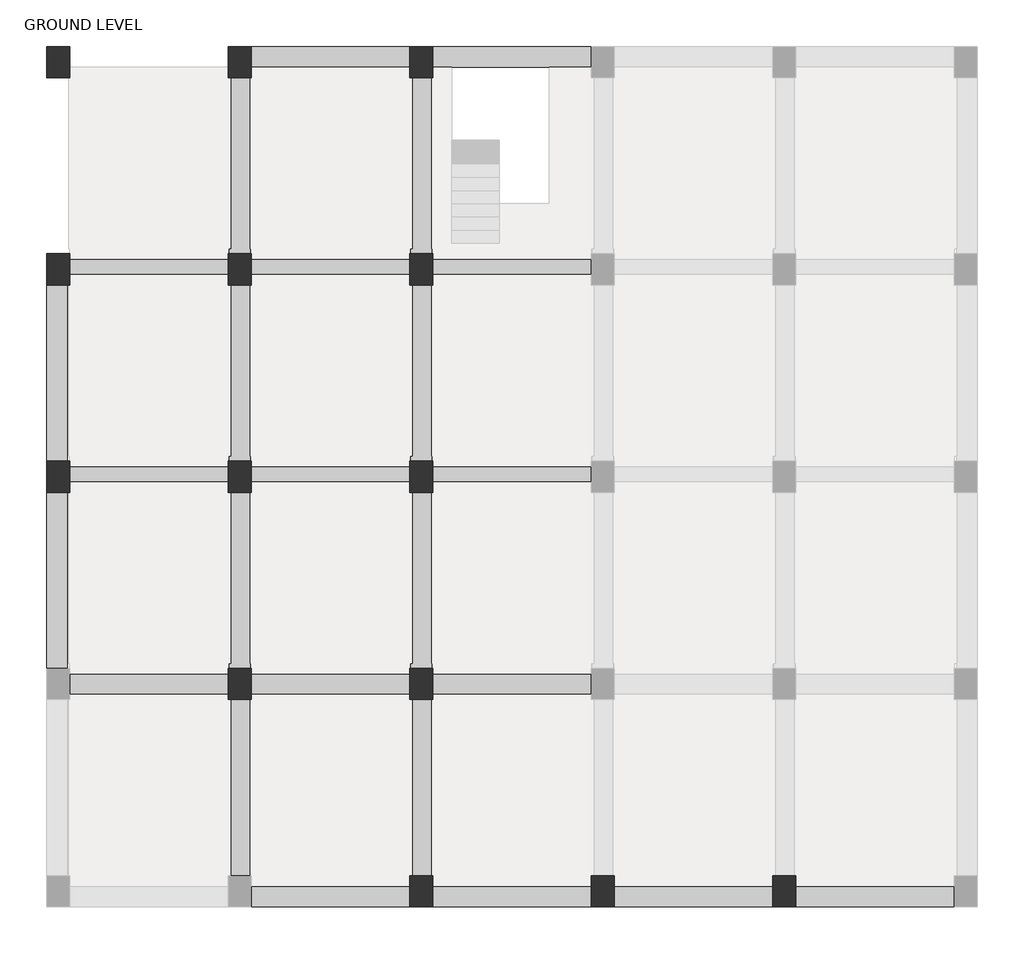
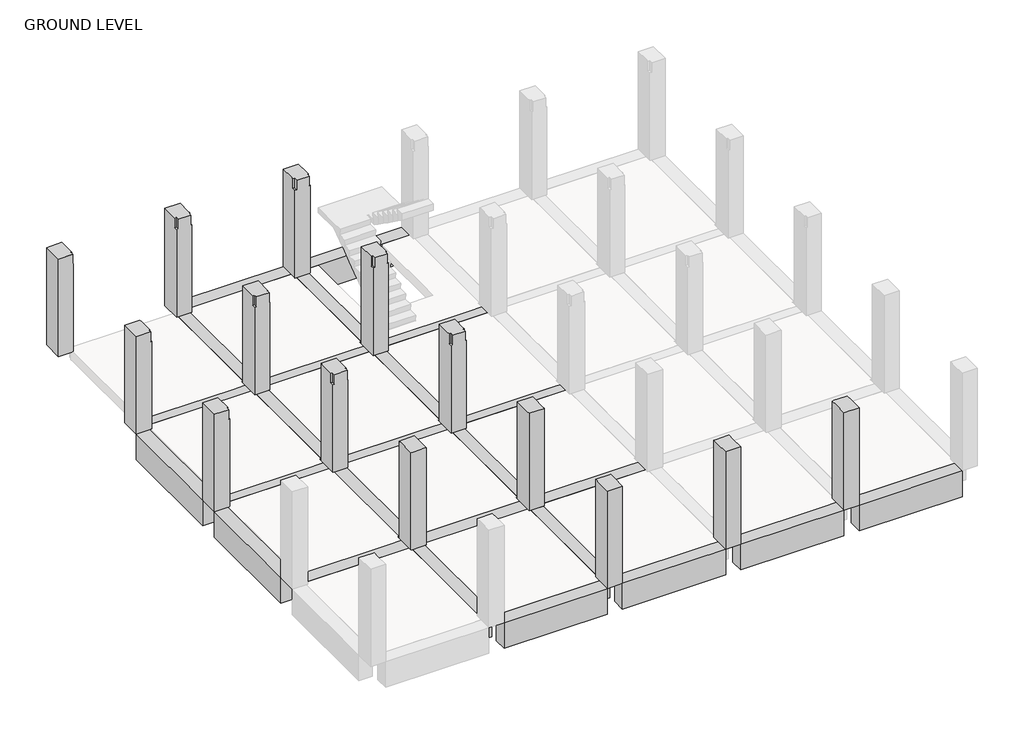
# One storey, part 2 of 3: 25 beams, 15 columns.
"""IFC4 building model written with IfcOpenShell, lengths in millimetres."""

from ifc_helpers import new_model, si_unit, frame, origin, place, context, project, spatial, polyline, outline, extrude, faceted_brep, element, save

model = new_model("IFC4")

# Units and contexts
model_context = context("Model", 3, world=origin())
ifc_project = project(units=[si_unit("LENGTHUNIT", "METRE", prefix="MILLI")], contexts=[model_context])

# Site, building, storey
site = spatial("IfcSite", under=ifc_project)
building = spatial("IfcBuilding", under=site)
storey = spatial("IfcBuildingStorey", under=building, Name="GROUND LEVEL", Elevation=0.0)

# Beams
placement = place(None, origin())
element("IfcBeam", 1, ObjectType="M_Concrete-Rectangular Beam : 400 x 800mm", at=placement, inside=storey, context=model_context, shape_type="Brep", body=[
    faceted_brep([(4855.1115906, 3503.1212443, 0.0), (4855.1115906, 3103.1212443, 0.0), (7905.1115906, 3103.1212443, 0.0), (7905.1115906, 3503.1212443, 0.0), (4855.1115906, 3503.1212443, -800.0), (4855.1115906, 3503.1212443, -300.0), (7905.1115906, 3503.1212443, -300.0), (7905.1115906, 3503.1212443, -800.0), (4855.1115906, 3103.1212443, -800.0), (7905.1115906, 3103.1212443, -800.0)], [[[0, 1, 2, 3]], [[4, 5, 0, 3, 6, 7]], [[8, 4, 7, 9]], [[1, 8, 9, 2]], [[1, 0, 5, 4, 8]], [[3, 2, 9, 7, 6]]]),
])
element("IfcBeam", 2, ObjectType="M_Concrete-Rectangular Beam : 400 x 800mm", at=placement, inside=storey, context=model_context, shape_type="Brep", body=[
    faceted_brep([(1355.1115906, 3503.1212443, 0.0), (1355.1115906, 3103.1212443, 0.0), (4405.1115906, 3103.1212443, 0.0), (4405.1115906, 3503.1212443, 0.0), (1355.1115906, 3503.1212443, -800.0), (1355.1115906, 3503.1212443, -300.0), (4405.1115906, 3503.1212443, -300.0), (4405.1115906, 3503.1212443, -800.0), (1355.1115906, 3103.1212443, -800.0), (4405.1115906, 3103.1212443, -800.0)], [[[0, 1, 2, 3]], [[4, 5, 0, 3, 6, 7]], [[8, 4, 7, 9]], [[1, 8, 9, 2]], [[1, 0, 5, 4, 8]], [[3, 2, 9, 7, 6]]]),
])
element("IfcBeam", 3, ObjectType="M_Concrete-Rectangular Beam : 400 x 800mm", at=placement, inside=storey, context=model_context, shape_type="Brep", body=[
    faceted_brep([(-2144.8884094, 3503.1212443, 0.0), (-2144.8884094, 3103.1212443, 0.0), (905.1115906, 3103.1212443, 0.0), (905.1115906, 3503.1212443, 0.0), (-2144.8884094, 3503.1212443, -800.0), (-2144.8884094, 3503.1212443, -300.0), (905.1115906, 3503.1212443, -300.0), (905.1115906, 3503.1212443, -800.0), (-2144.8884094, 3103.1212443, -800.0), (905.1115906, 3103.1212443, -800.0)], [[[0, 1, 2, 3]], [[4, 5, 0, 3, 6, 7]], [[8, 4, 7, 9]], [[1, 8, 9, 2]], [[1, 0, 5, 4, 8]], [[3, 2, 9, 7, 6]]]),
])
element("IfcBeam", 4, ObjectType="M_Concrete-Rectangular Beam : 400 x 800mm", at=placement, inside=storey, context=model_context, shape_type="Brep", body=[
    faceted_brep([(-5644.8884094, 3503.1212443, 0.0), (-5644.8884094, 3103.1212443, 0.0), (-2594.8884094, 3103.1212443, 0.0), (-2594.8884094, 3503.1212443, 0.0), (-5644.8884094, 3503.1212443, -800.0), (-5644.8884094, 3503.1212443, -300.0), (-2594.8884094, 3503.1212443, -300.0), (-2594.8884094, 3503.1212443, -800.0), (-5644.8884094, 3103.1212443, -800.0), (-2594.8884094, 3103.1212443, -800.0)], [[[0, 1, 2, 3]], [[4, 5, 0, 3, 6, 7]], [[8, 4, 7, 9]], [[1, 8, 9, 2]], [[1, 0, 5, 4, 8]], [[3, 2, 9, 7, 6]]]),
])
element("IfcBeam", 5, ObjectType="M_Concrete-Rectangular Beam : 400 x 800mm", at=placement, inside=storey, context=model_context, shape_type="SweptSolid", body=[
    extrude(outline(polyline([(-9594.8884094, 11103.1212443), (-9194.8884094, 11103.1212443), (-9194.8884094, 7703.1212443), (-9594.8884094, 7703.1212443), (-9594.8884094, 11103.1212443)])), frame((0.0, 0.0, -800.0), z_axis=(0.0, 0.0, 1.0), x_axis=(1.0, 0.0, 0.0)), (0.0, 0.0, 1.0), 800.0),
])
element("IfcBeam", 6, ObjectType="M_Concrete-Rectangular Beam : 400 x 800mm", at=placement, inside=storey, context=model_context, shape_type="SweptSolid", body=[
    extrude(outline(polyline([(-9594.8884094, 15103.1212443), (-9194.8884094, 15103.1212443), (-9194.8884094, 11703.1212443), (-9594.8884094, 11703.1212443), (-9594.8884094, 15103.1212443)])), frame((0.0, 0.0, -800.0), z_axis=(0.0, 0.0, 1.0), x_axis=(1.0, 0.0, 0.0)), (0.0, 0.0, 1.0), 800.0),
])
element("IfcBeam", 7, ObjectType="M_Concrete-Rectangular Beam : 400 x 800mm", at=placement, inside=storey, context=model_context, shape_type="Brep", body=[
    faceted_brep([(-2594.8884094, 19303.1212443, 0.0), (-2594.8884094, 19703.1212443, 0.0), (-5644.8884094, 19703.1212443, 0.0), (-5644.8884094, 19303.1212443, 0.0), (-2594.8884094, 19303.1212443, -800.0), (-2594.8884094, 19303.1212443, -300.0), (-5644.8884094, 19303.1212443, -300.0), (-5644.8884094, 19303.1212443, -800.0), (-2594.8884094, 19703.1212443, -800.0), (-5644.8884094, 19703.1212443, -800.0)], [[[0, 1, 2, 3]], [[4, 5, 0, 3, 6, 7]], [[8, 4, 7, 9]], [[1, 8, 9, 2]], [[1, 0, 5, 4, 8]], [[3, 2, 9, 7, 6]]]),
])
element("IfcBeam", 8, ObjectType="M_Concrete-Rectangular Beam : 400 x 800mm", at=placement, inside=storey, context=model_context, shape_type="Brep", body=[
    faceted_brep([(-2144.8884094, 19703.1212443, 0.0), (-2144.8884094, 19303.1212443, 0.0), (-1784.8884094, 19303.1212443, 0.0), (94.7115906, 19303.1212443, 0.0), (905.1115906, 19303.1212443, 0.0), (905.1115906, 19703.1212443, 0.0), (-2144.8884094, 19303.1212443, -300.0), (-2144.8884094, 19303.1212443, -800.0), (905.1115906, 19303.1212443, -800.0), (905.1115906, 19303.1212443, -300.0), (-2144.8884094, 19703.1212443, -800.0), (905.1115906, 19703.1212443, -800.0)], [[[0, 1, 2, 3, 4, 5]], [[1, 6, 7, 8, 9, 4, 3, 2]], [[7, 10, 11, 8]], [[10, 0, 5, 11]], [[1, 0, 10, 7, 6]], [[5, 4, 9, 8, 11]]]),
])
element("IfcBeam", 9, ObjectType="M_Concrete-Rectangular Beam : 400 x 800mm", at=placement, inside=storey, context=model_context, shape_type="Brep", body=[
    faceted_brep([(-5669.8884094, 15703.1212443, 0.0), (-5669.8884094, 15803.1212443, 0.0), (-5669.8884094, 19103.1212443, 0.0), (-6044.8884094, 19103.1212443, 0.0), (-6044.8884094, 15803.1212443, 0.0), (-6069.8884094, 15803.1212443, 0.0), (-6069.8884094, 15703.1212443, 0.0), (-6069.8884094, 19103.1212443, -800.0), (-6069.8884094, 15703.1212443, -800.0), (-6069.8884094, 15803.1212443, -300.0), (-6069.8884094, 19103.1212443, -300.0), (-5669.8884094, 19103.1212443, -800.0), (-5669.8884094, 15703.1212443, -800.0), (-6044.8884094, 19103.1212443, -300.0), (-6044.8884094, 15803.1212443, -300.0)], [[[0, 1, 2, 3, 4, 5, 6]], [[7, 8, 6, 5, 9, 10]], [[7, 11, 12, 8]], [[11, 2, 1, 0, 12]], [[11, 7, 10, 13, 3, 2]], [[0, 6, 8, 12]], [[9, 14, 13, 10]], [[14, 4, 3, 13]], [[4, 14, 9, 5]]]),
])
element("IfcBeam", 10, ObjectType="M_Concrete-Rectangular Beam : 400 x 800mm", at=placement, inside=storey, context=model_context, shape_type="Brep", body=[
    faceted_brep([(-5669.8884094, 11703.1212443, 0.0), (-5669.8884094, 11803.1212443, 0.0), (-5669.8884094, 15103.1212443, 0.0), (-6044.8884094, 15103.1212443, 0.0), (-6044.8884094, 11803.1212443, 0.0), (-6069.8884094, 11803.1212443, 0.0), (-6069.8884094, 11703.1212443, 0.0), (-6069.8884094, 15103.1212443, -800.0), (-6069.8884094, 11703.1212443, -800.0), (-6069.8884094, 11803.1212443, -300.0), (-6069.8884094, 15103.1212443, -300.0), (-5669.8884094, 15103.1212443, -800.0), (-5669.8884094, 11703.1212443, -800.0), (-6044.8884094, 15103.1212443, -300.0), (-6044.8884094, 11803.1212443, -300.0)], [[[0, 1, 2, 3, 4, 5, 6]], [[7, 8, 6, 5, 9, 10]], [[7, 11, 12, 8]], [[11, 2, 1, 0, 12]], [[11, 7, 10, 13, 3, 2]], [[0, 6, 8, 12]], [[9, 14, 13, 10]], [[14, 4, 3, 13]], [[4, 14, 9, 5]]]),
])
element("IfcBeam", 11, ObjectType="M_Concrete-Rectangular Beam : 400 x 800mm", at=placement, inside=storey, context=model_context, shape_type="Brep", body=[
    faceted_brep([(-5669.8884094, 7703.1212443, 0.0), (-5669.8884094, 7803.1212443, 0.0), (-5669.8884094, 11103.1212443, 0.0), (-6044.8884094, 11103.1212443, 0.0), (-6044.8884094, 7803.1212443, 0.0), (-6069.8884094, 7803.1212443, 0.0), (-6069.8884094, 7703.1212443, 0.0), (-6069.8884094, 11103.1212443, -800.0), (-6069.8884094, 7703.1212443, -800.0), (-6069.8884094, 7803.1212443, -300.0), (-6069.8884094, 11103.1212443, -300.0), (-5669.8884094, 11103.1212443, -800.0), (-5669.8884094, 7703.1212443, -800.0), (-6044.8884094, 11103.1212443, -300.0), (-6044.8884094, 7803.1212443, -300.0)], [[[0, 1, 2, 3, 4, 5, 6]], [[7, 8, 6, 5, 9, 10]], [[8, 7, 11, 12]], [[2, 1, 0, 12, 11]], [[2, 11, 7, 10, 13, 3]], [[0, 6, 8, 12]], [[9, 14, 13, 10]], [[14, 4, 3, 13]], [[4, 14, 9, 5]]]),
])
element("IfcBeam", 12, ObjectType="M_Concrete-Rectangular Beam : 400 x 800mm", at=placement, inside=storey, context=model_context, shape_type="Brep", body=[
    faceted_brep([(-5669.8884094, 3703.1212443, 0.0), (-5669.8884094, 7103.1212443, 0.0), (-6044.8884094, 7103.1212443, 0.0), (-6044.8884094, 3703.1212443, 0.0), (-6069.8884094, 7103.1212443, -800.0), (-6069.8884094, 3703.1212443, -800.0), (-6069.8884094, 3703.1212443, -300.0), (-6069.8884094, 7103.1212443, -300.0), (-5669.8884094, 7103.1212443, -800.0), (-5669.8884094, 3703.1212443, -800.0), (-5669.8884094, 7103.1212443, -300.0), (-5669.8884094, 3703.1212443, -300.0), (-6044.8884094, 7103.1212443, -300.0), (-6044.8884094, 3703.1212443, -300.0)], [[[0, 1, 2, 3]], [[4, 5, 6, 7]], [[4, 8, 9, 5]], [[8, 10, 1, 0, 11, 9]], [[8, 4, 7, 12, 2, 1, 10]], [[5, 9, 11, 0, 3, 13, 6]], [[13, 12, 7, 6]], [[12, 13, 3, 2]]]),
])
element("IfcBeam", 13, ObjectType="M_Concrete-Rectangular Beam : 400 x 800mm", at=placement, inside=storey, context=model_context, shape_type="Brep", body=[
    faceted_brep([(-2169.8884094, 15703.1212443, 0.0), (-2169.8884094, 15803.1212443, 0.0), (-2169.8884094, 19103.1212443, 0.0), (-2544.8884094, 19103.1212443, 0.0), (-2544.8884094, 15803.1212443, 0.0), (-2569.8884094, 15803.1212443, 0.0), (-2569.8884094, 15703.1212443, 0.0), (-2569.8884094, 19103.1212443, -800.0), (-2569.8884094, 15703.1212443, -800.0), (-2569.8884094, 15803.1212443, -300.0), (-2569.8884094, 19103.1212443, -300.0), (-2169.8884094, 19103.1212443, -800.0), (-2169.8884094, 15703.1212443, -800.0), (-2544.8884094, 19103.1212443, -300.0), (-2544.8884094, 15803.1212443, -300.0)], [[[0, 1, 2, 3, 4, 5, 6]], [[7, 8, 6, 5, 9, 10]], [[7, 11, 12, 8]], [[11, 2, 1, 0, 12]], [[11, 7, 10, 13, 3, 2]], [[0, 6, 8, 12]], [[9, 14, 13, 10]], [[14, 4, 3, 13]], [[4, 14, 9, 5]]]),
])
element("IfcBeam", 14, ObjectType="M_Concrete-Rectangular Beam : 400 x 800mm", at=placement, inside=storey, context=model_context, shape_type="Brep", body=[
    faceted_brep([(-2169.8884094, 11703.1212443, 0.0), (-2169.8884094, 11803.1212443, 0.0), (-2169.8884094, 15103.1212443, 0.0), (-2544.8884094, 15103.1212443, 0.0), (-2544.8884094, 11803.1212443, 0.0), (-2569.8884094, 11803.1212443, 0.0), (-2569.8884094, 11703.1212443, 0.0), (-2569.8884094, 15103.1212443, -800.0), (-2569.8884094, 11703.1212443, -800.0), (-2569.8884094, 11803.1212443, -300.0), (-2569.8884094, 15103.1212443, -300.0), (-2169.8884094, 15103.1212443, -800.0), (-2169.8884094, 11703.1212443, -800.0), (-2544.8884094, 15103.1212443, -300.0), (-2544.8884094, 11803.1212443, -300.0)], [[[0, 1, 2, 3, 4, 5, 6]], [[7, 8, 6, 5, 9, 10]], [[8, 7, 11, 12]], [[2, 1, 0, 12, 11]], [[2, 11, 7, 10, 13, 3]], [[0, 6, 8, 12]], [[9, 14, 13, 10]], [[14, 4, 3, 13]], [[4, 14, 9, 5]]]),
])
element("IfcBeam", 15, ObjectType="M_Concrete-Rectangular Beam : 400 x 800mm", at=placement, inside=storey, context=model_context, shape_type="Brep", body=[
    faceted_brep([(-2169.8884094, 7703.1212443, 0.0), (-2169.8884094, 7803.1212443, 0.0), (-2169.8884094, 11103.1212443, 0.0), (-2544.8884094, 11103.1212443, 0.0), (-2544.8884094, 7803.1212443, 0.0), (-2569.8884094, 7803.1212443, 0.0), (-2569.8884094, 7703.1212443, 0.0), (-2569.8884094, 11103.1212443, -800.0), (-2569.8884094, 7703.1212443, -800.0), (-2569.8884094, 7803.1212443, -300.0), (-2569.8884094, 11103.1212443, -300.0), (-2169.8884094, 11103.1212443, -800.0), (-2169.8884094, 7703.1212443, -800.0), (-2544.8884094, 11103.1212443, -300.0), (-2544.8884094, 7803.1212443, -300.0)], [[[0, 1, 2, 3, 4, 5, 6]], [[7, 8, 6, 5, 9, 10]], [[7, 11, 12, 8]], [[11, 2, 1, 0, 12]], [[2, 11, 7, 10, 13, 3]], [[0, 6, 8, 12]], [[9, 14, 13, 10]], [[14, 4, 3, 13]], [[4, 14, 9, 5]]]),
])
element("IfcBeam", 16, ObjectType="M_Concrete-Rectangular Beam : 400 x 800mm", at=placement, inside=storey, context=model_context, shape_type="Brep", body=[
    faceted_brep([(-2169.8884094, 3703.1212443, 0.0), (-2169.8884094, 7103.1212443, 0.0), (-2544.8884094, 7103.1212443, 0.0), (-2544.8884094, 3703.1212443, 0.0), (-2569.8884094, 7103.1212443, -800.0), (-2569.8884094, 3703.1212443, -800.0), (-2569.8884094, 3703.1212443, -300.0), (-2569.8884094, 7103.1212443, -300.0), (-2169.8884094, 7103.1212443, -800.0), (-2169.8884094, 3703.1212443, -800.0), (-2169.8884094, 7103.1212443, -300.0), (-2169.8884094, 3703.1212443, -300.0), (-2544.8884094, 7103.1212443, -300.0), (-2544.8884094, 3703.1212443, -300.0)], [[[0, 1, 2, 3]], [[4, 5, 6, 7]], [[4, 8, 9, 5]], [[8, 10, 1, 0, 11, 9]], [[8, 4, 7, 12, 2, 1, 10]], [[5, 9, 11, 0, 3, 13, 6]], [[13, 12, 7, 6]], [[12, 13, 3, 2]]]),
])
element("IfcBeam", 17, ObjectType="M_Concrete-Rectangular Beam : 400 x 800mm", at=placement, inside=storey, context=model_context, shape_type="Brep", body=[
    faceted_brep([(-6094.8884094, 15603.1212443, 0.0), (-9144.8884094, 15603.1212443, 0.0), (-9144.8884094, 15303.1212443, 0.0), (-6094.8884094, 15303.1212443, 0.0), (-9144.8884094, 15203.1212443, -800.0), (-6094.8884094, 15203.1212443, -800.0), (-6094.8884094, 15203.1212443, -300.0), (-9144.8884094, 15203.1212443, -300.0), (-9144.8884094, 15603.1212443, -800.0), (-6094.8884094, 15603.1212443, -800.0), (-9144.8884094, 15603.1212443, -300.0), (-6094.8884094, 15603.1212443, -300.0), (-9144.8884094, 15303.1212443, -300.0), (-6094.8884094, 15303.1212443, -300.0)], [[[0, 1, 2, 3]], [[4, 5, 6, 7]], [[4, 8, 9, 5]], [[8, 10, 1, 0, 11, 9]], [[8, 4, 7, 12, 2, 1, 10]], [[5, 9, 11, 0, 3, 13, 6]], [[13, 12, 7, 6]], [[12, 13, 3, 2]]]),
])
element("IfcBeam", 18, ObjectType="M_Concrete-Rectangular Beam : 400 x 800mm", at=placement, inside=storey, context=model_context, shape_type="Brep", body=[
    faceted_brep([(-2594.8884094, 15603.1212443, 0.0), (-5644.8884094, 15603.1212443, 0.0), (-5644.8884094, 15303.1212443, 0.0), (-2594.8884094, 15303.1212443, 0.0), (-5644.8884094, 15203.1212443, -800.0), (-2594.8884094, 15203.1212443, -800.0), (-2594.8884094, 15203.1212443, -300.0), (-5644.8884094, 15203.1212443, -300.0), (-5644.8884094, 15603.1212443, -800.0), (-2594.8884094, 15603.1212443, -800.0), (-5644.8884094, 15603.1212443, -300.0), (-2594.8884094, 15603.1212443, -300.0), (-5644.8884094, 15303.1212443, -300.0), (-2594.8884094, 15303.1212443, -300.0)], [[[0, 1, 2, 3]], [[4, 5, 6, 7]], [[4, 8, 9, 5]], [[8, 10, 1, 0, 11, 9]], [[8, 4, 7, 12, 2, 1, 10]], [[5, 9, 11, 0, 3, 13, 6]], [[13, 12, 7, 6]], [[12, 13, 3, 2]]]),
])
element("IfcBeam", 19, ObjectType="M_Concrete-Rectangular Beam : 400 x 800mm", at=placement, inside=storey, context=model_context, shape_type="Brep", body=[
    faceted_brep([(905.1115906, 15603.1212443, 0.0), (-2144.8884094, 15603.1212443, 0.0), (-2144.8884094, 15303.1212443, 0.0), (905.1115906, 15303.1212443, 0.0), (-2144.8884094, 15603.1212443, -800.0), (-2144.8884094, 15603.1212443, -300.0), (905.1115906, 15603.1212443, -300.0), (905.1115906, 15603.1212443, -800.0), (-2144.8884094, 15203.1212443, -800.0), (905.1115906, 15203.1212443, -800.0), (905.1115906, 15203.1212443, -300.0), (-2144.8884094, 15203.1212443, -300.0), (-2144.8884094, 15303.1212443, -300.0), (905.1115906, 15303.1212443, -300.0)], [[[0, 1, 2, 3]], [[4, 5, 1, 0, 6, 7]], [[8, 4, 7, 9]], [[8, 9, 10, 11]], [[1, 5, 4, 8, 11, 12, 2]], [[7, 6, 0, 3, 13, 10, 9]], [[13, 12, 11, 10]], [[12, 13, 3, 2]]]),
])
element("IfcBeam", 20, ObjectType="M_Concrete-Rectangular Beam : 400 x 800mm", at=placement, inside=storey, context=model_context, shape_type="Brep", body=[
    faceted_brep([(905.1115906, 11603.1212443, 0.0), (-2144.8884094, 11603.1212443, 0.0), (-2144.8884094, 11303.1212443, 0.0), (905.1115906, 11303.1212443, 0.0), (-2144.8884094, 11603.1212443, -800.0), (-2144.8884094, 11603.1212443, -300.0), (905.1115906, 11603.1212443, -300.0), (905.1115906, 11603.1212443, -800.0), (-2144.8884094, 11203.1212443, -800.0), (905.1115906, 11203.1212443, -800.0), (905.1115906, 11203.1212443, -300.0), (-2144.8884094, 11203.1212443, -300.0), (-2144.8884094, 11303.1212443, -300.0), (905.1115906, 11303.1212443, -300.0)], [[[0, 1, 2, 3]], [[4, 5, 1, 0, 6, 7]], [[8, 4, 7, 9]], [[8, 9, 10, 11]], [[1, 5, 4, 8, 11, 12, 2]], [[7, 6, 0, 3, 13, 10, 9]], [[13, 12, 11, 10]], [[12, 13, 3, 2]]]),
])
element("IfcBeam", 21, ObjectType="M_Concrete-Rectangular Beam : 400 x 800mm", at=placement, inside=storey, context=model_context, shape_type="Brep", body=[
    faceted_brep([(-2594.8884094, 11603.1212443, 0.0), (-5644.8884094, 11603.1212443, 0.0), (-5644.8884094, 11303.1212443, 0.0), (-2594.8884094, 11303.1212443, 0.0), (-5644.8884094, 11603.1212443, -800.0), (-5644.8884094, 11603.1212443, -300.0), (-2594.8884094, 11603.1212443, -300.0), (-2594.8884094, 11603.1212443, -800.0), (-5644.8884094, 11203.1212443, -800.0), (-2594.8884094, 11203.1212443, -800.0), (-2594.8884094, 11203.1212443, -300.0), (-5644.8884094, 11203.1212443, -300.0), (-5644.8884094, 11303.1212443, -300.0), (-2594.8884094, 11303.1212443, -300.0)], [[[0, 1, 2, 3]], [[4, 5, 1, 0, 6, 7]], [[8, 4, 7, 9]], [[8, 9, 10, 11]], [[1, 5, 4, 8, 11, 12, 2]], [[7, 6, 0, 3, 13, 10, 9]], [[13, 12, 11, 10]], [[12, 13, 3, 2]]]),
])
element("IfcBeam", 22, ObjectType="M_Concrete-Rectangular Beam : 400 x 800mm", at=placement, inside=storey, context=model_context, shape_type="Brep", body=[
    faceted_brep([(-6094.8884094, 11603.1212443, 0.0), (-9144.8884094, 11603.1212443, 0.0), (-9144.8884094, 11303.1212443, 0.0), (-6094.8884094, 11303.1212443, 0.0), (-9144.8884094, 11603.1212443, -800.0), (-9144.8884094, 11603.1212443, -300.0), (-6094.8884094, 11603.1212443, -300.0), (-6094.8884094, 11603.1212443, -800.0), (-9144.8884094, 11203.1212443, -800.0), (-6094.8884094, 11203.1212443, -800.0), (-6094.8884094, 11203.1212443, -300.0), (-9144.8884094, 11203.1212443, -300.0), (-9144.8884094, 11303.1212443, -300.0), (-6094.8884094, 11303.1212443, -300.0)], [[[0, 1, 2, 3]], [[4, 5, 1, 0, 6, 7]], [[8, 4, 7, 9]], [[8, 9, 10, 11]], [[1, 5, 4, 8, 11, 12, 2]], [[7, 6, 0, 3, 13, 10, 9]], [[13, 12, 11, 10]], [[12, 13, 3, 2]]]),
])
element("IfcBeam", 23, ObjectType="M_Concrete-Rectangular Beam : 400 x 800mm", at=placement, inside=storey, context=model_context, shape_type="Brep", body=[
    faceted_brep([(-9144.8884094, 7603.1212443, 0.0), (-9144.8884094, 7203.1212443, 0.0), (-6094.8884094, 7203.1212443, 0.0), (-6094.8884094, 7603.1212443, 0.0), (-9144.8884094, 7203.1212443, -300.0), (-9144.8884094, 7203.1212443, -800.0), (-6094.8884094, 7203.1212443, -800.0), (-6094.8884094, 7203.1212443, -300.0), (-9144.8884094, 7603.1212443, -800.0), (-6094.8884094, 7603.1212443, -800.0), (-9144.8884094, 7603.1212443, -300.0), (-6094.8884094, 7603.1212443, -300.0)], [[[0, 1, 2, 3]], [[1, 4, 5, 6, 7, 2]], [[5, 8, 9, 6]], [[8, 10, 0, 3, 11, 9]], [[1, 0, 10, 8, 5, 4]], [[3, 2, 7, 6, 9, 11]]]),
])
element("IfcBeam", 24, ObjectType="M_Concrete-Rectangular Beam : 400 x 800mm", at=placement, inside=storey, context=model_context, shape_type="Brep", body=[
    faceted_brep([(-5644.8884094, 7603.1212443, 0.0), (-5644.8884094, 7203.1212443, 0.0), (-2594.8884094, 7203.1212443, 0.0), (-2594.8884094, 7603.1212443, 0.0), (-5644.8884094, 7203.1212443, -300.0), (-5644.8884094, 7203.1212443, -800.0), (-2594.8884094, 7203.1212443, -800.0), (-2594.8884094, 7203.1212443, -300.0), (-5644.8884094, 7603.1212443, -800.0), (-2594.8884094, 7603.1212443, -800.0), (-5644.8884094, 7603.1212443, -300.0), (-2594.8884094, 7603.1212443, -300.0)], [[[0, 1, 2, 3]], [[1, 4, 5, 6, 7, 2]], [[5, 8, 9, 6]], [[8, 10, 0, 3, 11, 9]], [[1, 0, 10, 8, 5, 4]], [[3, 2, 7, 6, 9, 11]]]),
])
element("IfcBeam", 25, ObjectType="M_Concrete-Rectangular Beam : 400 x 800mm", at=placement, inside=storey, context=model_context, shape_type="Brep", body=[
    faceted_brep([(-2144.8884094, 7603.1212443, 0.0), (-2144.8884094, 7203.1212443, 0.0), (905.1115906, 7203.1212443, 0.0), (905.1115906, 7603.1212443, 0.0), (-2144.8884094, 7203.1212443, -300.0), (-2144.8884094, 7203.1212443, -800.0), (905.1115906, 7203.1212443, -800.0), (905.1115906, 7203.1212443, -300.0), (-2144.8884094, 7603.1212443, -800.0), (905.1115906, 7603.1212443, -800.0), (-2144.8884094, 7603.1212443, -300.0), (905.1115906, 7603.1212443, -300.0)], [[[0, 1, 2, 3]], [[1, 4, 5, 6, 7, 2]], [[5, 8, 9, 6]], [[8, 10, 0, 3, 11, 9]], [[1, 0, 10, 8, 5, 4]], [[3, 2, 7, 6, 9, 11]]]),
])

# Columns
element("IfcColumn", 26, ObjectType="M_Concrete-Rectangular-Column : 450 x 600mm", at=placement, inside=storey, context=model_context, shape_type="Brep", body=[
    faceted_brep([(-9144.8884094, 19703.1212443, 0.0), (-9144.8884094, 19103.1212443, 0.0), (-9594.8884094, 19103.1212443, 0.0), (-9594.8884094, 19703.1212443, 0.0), (-9144.8884094, 19703.1212443, 3048.0), (-9144.8884094, 19303.1212443, 3048.0), (-9144.8884094, 19203.1212443, 3048.0), (-9144.8884094, 19203.1212443, 2748.0), (-9144.8884094, 19103.1212443, 2748.0), (-9169.8884094, 19103.1212443, 2748.0), (-9169.8884094, 19103.1212443, 3048.0), (-9594.8884094, 19103.1212443, 3048.0), (-9594.8884094, 19703.1212443, 3048.0), (-9169.8884094, 19203.1212443, 3048.0), (-9169.8884094, 19203.1212443, 2748.0)], [[[0, 1, 2, 3]], [[1, 0, 4, 5, 6, 7, 8]], [[2, 1, 8, 9, 10, 11]], [[3, 2, 11, 12]], [[0, 3, 12, 4]], [[12, 11, 10, 13, 6, 5, 4]], [[7, 14, 9, 8]], [[14, 13, 10, 9]], [[14, 7, 6, 13]]]),
])
element("IfcColumn", 27, ObjectType="M_Concrete-Rectangular-Column : 450 x 600mm", at=placement, inside=storey, context=model_context, shape_type="Brep", body=[
    faceted_brep([(-5644.8884094, 19703.1212443, 0.0), (-5644.8884094, 19103.1212443, 0.0), (-6094.8884094, 19103.1212443, 0.0), (-6094.8884094, 19703.1212443, 0.0), (-5644.8884094, 19703.1212443, 3048.0), (-5644.8884094, 19303.1212443, 3048.0), (-5644.8884094, 19203.1212443, 3048.0), (-5644.8884094, 19203.1212443, 2748.0), (-5644.8884094, 19103.1212443, 2748.0), (-5669.8884094, 19103.1212443, 2748.0), (-5669.8884094, 19103.1212443, 3048.0), (-6044.8884094, 19103.1212443, 3048.0), (-6044.8884094, 19103.1212443, 2748.0), (-6094.8884094, 19103.1212443, 2748.0), (-6094.8884094, 19203.1212443, 2748.0), (-6094.8884094, 19203.1212443, 3048.0), (-6094.8884094, 19303.1212443, 3048.0), (-6094.8884094, 19703.1212443, 3048.0), (-6044.8884094, 19203.1212443, 3048.0), (-5669.8884094, 19203.1212443, 3048.0), (-5669.8884094, 19203.1212443, 2748.0), (-6044.8884094, 19203.1212443, 2748.0)], [[[0, 1, 2, 3]], [[1, 0, 4, 5, 6, 7, 8]], [[2, 1, 8, 9, 10, 11, 12, 13]], [[3, 2, 13, 14, 15, 16, 17]], [[0, 3, 17, 4]], [[4, 17, 16, 15, 18, 11, 10, 19, 6, 5]], [[7, 20, 9, 8]], [[20, 19, 10, 9]], [[20, 7, 6, 19]], [[21, 14, 13, 12]], [[18, 21, 12, 11]], [[14, 21, 18, 15]]]),
])
element("IfcColumn", 28, ObjectType="M_Concrete-Rectangular-Column : 450 x 600mm", at=placement, inside=storey, context=model_context, shape_type="Brep", body=[
    faceted_brep([(-2144.8884094, 19703.1212443, 0.0), (-2144.8884094, 19103.1212443, 0.0), (-2594.8884094, 19103.1212443, 0.0), (-2594.8884094, 19703.1212443, 0.0), (-2144.8884094, 19703.1212443, 3048.0), (-2144.8884094, 19303.1212443, 3048.0), (-2144.8884094, 19203.1212443, 3048.0), (-2144.8884094, 19203.1212443, 2748.0), (-2144.8884094, 19103.1212443, 2748.0), (-2169.8884094, 19103.1212443, 2748.0), (-2169.8884094, 19103.1212443, 3048.0), (-2544.8884094, 19103.1212443, 3048.0), (-2544.8884094, 19103.1212443, 2748.0), (-2594.8884094, 19103.1212443, 2748.0), (-2594.8884094, 19203.1212443, 2748.0), (-2594.8884094, 19203.1212443, 3048.0), (-2594.8884094, 19303.1212443, 3048.0), (-2594.8884094, 19703.1212443, 3048.0), (-2544.8884094, 19203.1212443, 3048.0), (-2169.8884094, 19203.1212443, 3048.0), (-2169.8884094, 19203.1212443, 2748.0), (-2544.8884094, 19203.1212443, 2748.0)], [[[0, 1, 2, 3]], [[1, 0, 4, 5, 6, 7, 8]], [[2, 1, 8, 9, 10, 11, 12, 13]], [[3, 2, 13, 14, 15, 16, 17]], [[0, 3, 17, 4]], [[4, 17, 16, 15, 18, 11, 10, 19, 6, 5]], [[7, 20, 9, 8]], [[20, 19, 10, 9]], [[20, 7, 6, 19]], [[21, 14, 13, 12]], [[18, 21, 12, 11]], [[14, 21, 18, 15]]]),
])
element("IfcColumn", 29, ObjectType="M_Concrete-Rectangular-Column : 450 x 600mm", at=placement, inside=storey, context=model_context, shape_type="Brep", body=[
    faceted_brep([(-9144.8884094, 15703.1212443, 0.0), (-9144.8884094, 15103.1212443, 0.0), (-9594.8884094, 15103.1212443, 0.0), (-9594.8884094, 15703.1212443, 0.0), (-9144.8884094, 15703.1212443, 2748.0), (-9144.8884094, 15703.1212443, 3048.0), (-9144.8884094, 15603.1212443, 3048.0), (-9144.8884094, 15303.1212443, 3048.0), (-9144.8884094, 15203.1212443, 3048.0), (-9144.8884094, 15203.1212443, 2748.0), (-9144.8884094, 15103.1212443, 2748.0), (-9169.8884094, 15103.1212443, 2748.0), (-9169.8884094, 15103.1212443, 3048.0), (-9594.8884094, 15103.1212443, 3048.0), (-9594.8884094, 15703.1212443, 3048.0), (-9169.8884094, 15203.1212443, 3048.0), (-9169.8884094, 15203.1212443, 2748.0)], [[[0, 1, 2, 3]], [[1, 0, 4, 5, 6, 7, 8, 9, 10]], [[2, 1, 10, 11, 12, 13]], [[3, 2, 13, 14]], [[0, 3, 14, 5, 4]], [[14, 13, 12, 15, 8, 7, 6, 5]], [[9, 16, 11, 10]], [[16, 15, 12, 11]], [[16, 9, 8, 15]]]),
])
element("IfcColumn", 30, ObjectType="M_Concrete-Rectangular-Column : 450 x 600mm", at=placement, inside=storey, context=model_context, shape_type="Brep", body=[
    faceted_brep([(-5644.8884094, 15703.1212443, 0.0), (-5644.8884094, 15103.1212443, 0.0), (-6094.8884094, 15103.1212443, 0.0), (-6094.8884094, 15703.1212443, 0.0), (-5644.8884094, 15703.1212443, 2748.0), (-5644.8884094, 15703.1212443, 3048.0), (-5644.8884094, 15603.1212443, 3048.0), (-5644.8884094, 15303.1212443, 3048.0), (-5644.8884094, 15203.1212443, 3048.0), (-5644.8884094, 15203.1212443, 2748.0), (-5644.8884094, 15103.1212443, 2748.0), (-5669.8884094, 15103.1212443, 2748.0), (-5669.8884094, 15103.1212443, 3048.0), (-6044.8884094, 15103.1212443, 3048.0), (-6044.8884094, 15103.1212443, 2748.0), (-6094.8884094, 15103.1212443, 2748.0), (-6094.8884094, 15203.1212443, 2748.0), (-6094.8884094, 15203.1212443, 3048.0), (-6094.8884094, 15303.1212443, 3048.0), (-6094.8884094, 15603.1212443, 3048.0), (-6094.8884094, 15703.1212443, 3048.0), (-6094.8884094, 15703.1212443, 2748.0), (-6044.8884094, 15203.1212443, 3048.0), (-5669.8884094, 15203.1212443, 3048.0), (-6044.8884094, 15203.1212443, 2748.0), (-5669.8884094, 15203.1212443, 2748.0)], [[[0, 1, 2, 3]], [[1, 0, 4, 5, 6, 7, 8, 9, 10]], [[2, 1, 10, 11, 12, 13, 14, 15]], [[3, 2, 15, 16, 17, 18, 19, 20, 21]], [[0, 3, 21, 20, 5, 4]], [[5, 20, 19, 18, 17, 22, 13, 12, 23, 8, 7, 6]], [[24, 16, 15, 14]], [[22, 24, 14, 13]], [[16, 24, 22, 17]], [[9, 25, 11, 10]], [[25, 23, 12, 11]], [[25, 9, 8, 23]]]),
])
element("IfcColumn", 31, ObjectType="M_Concrete-Rectangular-Column : 450 x 600mm", at=placement, inside=storey, context=model_context, shape_type="Brep", body=[
    faceted_brep([(-2144.8884094, 15703.1212443, 0.0), (-2144.8884094, 15103.1212443, 0.0), (-2594.8884094, 15103.1212443, 0.0), (-2594.8884094, 15703.1212443, 0.0), (-2144.8884094, 15703.1212443, 2748.0), (-2144.8884094, 15703.1212443, 3048.0), (-2144.8884094, 15603.1212443, 3048.0), (-2144.8884094, 15303.1212443, 3048.0), (-2144.8884094, 15203.1212443, 3048.0), (-2144.8884094, 15203.1212443, 2748.0), (-2144.8884094, 15103.1212443, 2748.0), (-2169.8884094, 15103.1212443, 2748.0), (-2169.8884094, 15103.1212443, 3048.0), (-2544.8884094, 15103.1212443, 3048.0), (-2544.8884094, 15103.1212443, 2748.0), (-2594.8884094, 15103.1212443, 2748.0), (-2594.8884094, 15203.1212443, 2748.0), (-2594.8884094, 15203.1212443, 3048.0), (-2594.8884094, 15303.1212443, 3048.0), (-2594.8884094, 15603.1212443, 3048.0), (-2594.8884094, 15703.1212443, 3048.0), (-2594.8884094, 15703.1212443, 2748.0), (-2544.8884094, 15203.1212443, 3048.0), (-2169.8884094, 15203.1212443, 3048.0), (-2169.8884094, 15203.1212443, 2748.0), (-2544.8884094, 15203.1212443, 2748.0)], [[[0, 1, 2, 3]], [[1, 0, 4, 5, 6, 7, 8, 9, 10]], [[2, 1, 10, 11, 12, 13, 14, 15]], [[3, 2, 15, 16, 17, 18, 19, 20, 21]], [[0, 3, 21, 20, 5, 4]], [[5, 20, 19, 18, 17, 22, 13, 12, 23, 8, 7, 6]], [[9, 24, 11, 10]], [[24, 23, 12, 11]], [[24, 9, 8, 23]], [[25, 16, 15, 14]], [[22, 25, 14, 13]], [[16, 25, 22, 17]]]),
])
element("IfcColumn", 32, ObjectType="M_Concrete-Rectangular-Column : 450 x 600mm", at=placement, inside=storey, context=model_context, shape_type="Brep", body=[
    faceted_brep([(-9144.8884094, 11703.1212443, 0.0), (-9144.8884094, 11103.1212443, 0.0), (-9594.8884094, 11103.1212443, 0.0), (-9594.8884094, 11703.1212443, 0.0), (-9144.8884094, 11703.1212443, 2748.0), (-9144.8884094, 11703.1212443, 3048.0), (-9144.8884094, 11603.1212443, 3048.0), (-9144.8884094, 11303.1212443, 3048.0), (-9144.8884094, 11203.1212443, 3048.0), (-9144.8884094, 11203.1212443, 2748.0), (-9144.8884094, 11103.1212443, 2748.0), (-9169.8884094, 11103.1212443, 2748.0), (-9169.8884094, 11103.1212443, 3048.0), (-9594.8884094, 11103.1212443, 3048.0), (-9594.8884094, 11703.1212443, 3048.0), (-9169.8884094, 11203.1212443, 3048.0), (-9169.8884094, 11203.1212443, 2748.0)], [[[0, 1, 2, 3]], [[1, 0, 4, 5, 6, 7, 8, 9, 10]], [[2, 1, 10, 11, 12, 13]], [[3, 2, 13, 14]], [[0, 3, 14, 5, 4]], [[14, 13, 12, 15, 8, 7, 6, 5]], [[9, 16, 11, 10]], [[16, 15, 12, 11]], [[16, 9, 8, 15]]]),
])
element("IfcColumn", 33, ObjectType="M_Concrete-Rectangular-Column : 450 x 600mm", at=placement, inside=storey, context=model_context, shape_type="Brep", body=[
    faceted_brep([(-5644.8884094, 11703.1212443, 0.0), (-5644.8884094, 11103.1212443, 0.0), (-6094.8884094, 11103.1212443, 0.0), (-6094.8884094, 11703.1212443, 0.0), (-5644.8884094, 11703.1212443, 2748.0), (-5644.8884094, 11703.1212443, 3048.0), (-5644.8884094, 11603.1212443, 3048.0), (-5644.8884094, 11303.1212443, 3048.0), (-5644.8884094, 11203.1212443, 3048.0), (-5644.8884094, 11203.1212443, 2748.0), (-5644.8884094, 11103.1212443, 2748.0), (-5669.8884094, 11103.1212443, 2748.0), (-5669.8884094, 11103.1212443, 3048.0), (-6044.8884094, 11103.1212443, 3048.0), (-6044.8884094, 11103.1212443, 2748.0), (-6094.8884094, 11103.1212443, 2748.0), (-6094.8884094, 11203.1212443, 2748.0), (-6094.8884094, 11203.1212443, 3048.0), (-6094.8884094, 11303.1212443, 3048.0), (-6094.8884094, 11603.1212443, 3048.0), (-6094.8884094, 11703.1212443, 3048.0), (-6094.8884094, 11703.1212443, 2748.0), (-6044.8884094, 11203.1212443, 3048.0), (-5669.8884094, 11203.1212443, 3048.0), (-5669.8884094, 11203.1212443, 2748.0), (-6044.8884094, 11203.1212443, 2748.0)], [[[0, 1, 2, 3]], [[1, 0, 4, 5, 6, 7, 8, 9, 10]], [[2, 1, 10, 11, 12, 13, 14, 15]], [[3, 2, 15, 16, 17, 18, 19, 20, 21]], [[0, 3, 21, 20, 5, 4]], [[5, 20, 19, 18, 17, 22, 13, 12, 23, 8, 7, 6]], [[9, 24, 11, 10]], [[24, 23, 12, 11]], [[24, 9, 8, 23]], [[25, 16, 15, 14]], [[22, 25, 14, 13]], [[16, 25, 22, 17]]]),
])
element("IfcColumn", 34, ObjectType="M_Concrete-Rectangular-Column : 450 x 600mm", at=placement, inside=storey, context=model_context, shape_type="Brep", body=[
    faceted_brep([(-2144.8884094, 11703.1212443, 0.0), (-2144.8884094, 11103.1212443, 0.0), (-2594.8884094, 11103.1212443, 0.0), (-2594.8884094, 11703.1212443, 0.0), (-2144.8884094, 11703.1212443, 2748.0), (-2144.8884094, 11703.1212443, 3048.0), (-2144.8884094, 11603.1212443, 3048.0), (-2144.8884094, 11303.1212443, 3048.0), (-2144.8884094, 11203.1212443, 3048.0), (-2144.8884094, 11203.1212443, 2748.0), (-2144.8884094, 11103.1212443, 2748.0), (-2169.8884094, 11103.1212443, 2748.0), (-2169.8884094, 11103.1212443, 3048.0), (-2544.8884094, 11103.1212443, 3048.0), (-2544.8884094, 11103.1212443, 2748.0), (-2594.8884094, 11103.1212443, 2748.0), (-2594.8884094, 11203.1212443, 2748.0), (-2594.8884094, 11203.1212443, 3048.0), (-2594.8884094, 11303.1212443, 3048.0), (-2594.8884094, 11603.1212443, 3048.0), (-2594.8884094, 11703.1212443, 3048.0), (-2594.8884094, 11703.1212443, 2748.0), (-2544.8884094, 11203.1212443, 3048.0), (-2169.8884094, 11203.1212443, 3048.0), (-2169.8884094, 11203.1212443, 2748.0), (-2544.8884094, 11203.1212443, 2748.0)], [[[0, 1, 2, 3]], [[1, 0, 4, 5, 6, 7, 8, 9, 10]], [[2, 1, 10, 11, 12, 13, 14, 15]], [[3, 2, 15, 16, 17, 18, 19, 20, 21]], [[0, 3, 21, 20, 5, 4]], [[5, 20, 19, 18, 17, 22, 13, 12, 23, 8, 7, 6]], [[9, 24, 11, 10]], [[24, 23, 12, 11]], [[24, 9, 8, 23]], [[25, 16, 15, 14]], [[22, 25, 14, 13]], [[16, 25, 22, 17]]]),
])
element("IfcColumn", 35, ObjectType="M_Concrete-Rectangular-Column : 450 x 600mm", at=placement, inside=storey, context=model_context, shape_type="Brep", body=[
    faceted_brep([(-5644.8884094, 7703.1212443, 0.0), (-5644.8884094, 7103.1212443, 0.0), (-6094.8884094, 7103.1212443, 0.0), (-6094.8884094, 7703.1212443, 0.0), (-5644.8884094, 7703.1212443, 2748.0), (-5644.8884094, 7703.1212443, 3048.0), (-5644.8884094, 7603.1212443, 3048.0), (-5644.8884094, 7203.1212443, 3048.0), (-5644.8884094, 7103.1212443, 3048.0), (-5644.8884094, 7103.1212443, 2748.0), (-5669.8884094, 7103.1212443, 3048.0), (-6044.8884094, 7103.1212443, 3048.0), (-6094.8884094, 7103.1212443, 3048.0), (-6094.8884094, 7103.1212443, 2748.0), (-6094.8884094, 7203.1212443, 3048.0), (-6094.8884094, 7603.1212443, 3048.0), (-6094.8884094, 7703.1212443, 3048.0), (-6094.8884094, 7703.1212443, 2748.0)], [[[0, 1, 2, 3]], [[1, 0, 4, 5, 6, 7, 8, 9]], [[2, 1, 9, 8, 10, 11, 12, 13]], [[3, 2, 13, 12, 14, 15, 16, 17]], [[0, 3, 17, 16, 5, 4]], [[5, 16, 15, 14, 12, 11, 10, 8, 7, 6]]]),
])
element("IfcColumn", 36, ObjectType="M_Concrete-Rectangular-Column : 450 x 600mm", at=placement, inside=storey, context=model_context, shape_type="Brep", body=[
    faceted_brep([(-2144.8884094, 7703.1212443, 0.0), (-2144.8884094, 7103.1212443, 0.0), (-2594.8884094, 7103.1212443, 0.0), (-2594.8884094, 7703.1212443, 0.0), (-2144.8884094, 7703.1212443, 2748.0), (-2144.8884094, 7703.1212443, 3048.0), (-2144.8884094, 7603.1212443, 3048.0), (-2144.8884094, 7203.1212443, 3048.0), (-2144.8884094, 7103.1212443, 3048.0), (-2144.8884094, 7103.1212443, 2748.0), (-2169.8884094, 7103.1212443, 3048.0), (-2544.8884094, 7103.1212443, 3048.0), (-2594.8884094, 7103.1212443, 3048.0), (-2594.8884094, 7103.1212443, 2748.0), (-2594.8884094, 7203.1212443, 3048.0), (-2594.8884094, 7603.1212443, 3048.0), (-2594.8884094, 7703.1212443, 3048.0), (-2594.8884094, 7703.1212443, 2748.0)], [[[0, 1, 2, 3]], [[1, 0, 4, 5, 6, 7, 8, 9]], [[2, 1, 9, 8, 10, 11, 12, 13]], [[3, 2, 13, 12, 14, 15, 16, 17]], [[0, 3, 17, 16, 5, 4]], [[5, 16, 15, 14, 12, 11, 10, 8, 7, 6]]]),
])
element("IfcColumn", 37, ObjectType="M_Concrete-Rectangular-Column : 450 x 600mm", at=placement, inside=storey, context=model_context, shape_type="Brep", body=[
    faceted_brep([(-2144.8884094, 3703.1212443, 0.0), (-2144.8884094, 3103.1212443, 0.0), (-2594.8884094, 3103.1212443, 0.0), (-2594.8884094, 3703.1212443, 0.0), (-2144.8884094, 3703.1212443, 2748.0), (-2144.8884094, 3703.1212443, 3048.0), (-2144.8884094, 3503.1212443, 3048.0), (-2144.8884094, 3103.1212443, 3048.0), (-2594.8884094, 3103.1212443, 3048.0), (-2594.8884094, 3503.1212443, 3048.0), (-2594.8884094, 3703.1212443, 3048.0), (-2594.8884094, 3703.1212443, 2748.0), (-2544.8884094, 3703.1212443, 3048.0), (-2169.8884094, 3703.1212443, 3048.0)], [[[0, 1, 2, 3]], [[1, 0, 4, 5, 6, 7]], [[2, 1, 7, 8]], [[3, 2, 8, 9, 10, 11]], [[0, 3, 11, 10, 12, 13, 5, 4]], [[8, 7, 6, 5, 13, 12, 10, 9]]]),
])
element("IfcColumn", 38, ObjectType="M_Concrete-Rectangular-Column : 450 x 600mm", at=placement, inside=storey, context=model_context, shape_type="Brep", body=[
    faceted_brep([(1355.1115906, 3703.1212443, 0.0), (1355.1115906, 3103.1212443, 0.0), (905.1115906, 3103.1212443, 0.0), (905.1115906, 3703.1212443, 0.0), (1355.1115906, 3703.1212443, 2748.0), (1355.1115906, 3703.1212443, 3048.0), (1355.1115906, 3503.1212443, 3048.0), (1355.1115906, 3103.1212443, 3048.0), (905.1115906, 3103.1212443, 3048.0), (905.1115906, 3503.1212443, 3048.0), (905.1115906, 3703.1212443, 3048.0), (905.1115906, 3703.1212443, 2748.0), (955.1115906, 3703.1212443, 3048.0), (1330.1115906, 3703.1212443, 3048.0)], [[[0, 1, 2, 3]], [[1, 0, 4, 5, 6, 7]], [[2, 1, 7, 8]], [[3, 2, 8, 9, 10, 11]], [[0, 3, 11, 10, 12, 13, 5, 4]], [[8, 7, 6, 5, 13, 12, 10, 9]]]),
])
element("IfcColumn", 39, ObjectType="M_Concrete-Rectangular-Column : 450 x 600mm", at=placement, inside=storey, context=model_context, shape_type="Brep", body=[
    faceted_brep([(4855.1115906, 3703.1212443, 0.0), (4855.1115906, 3103.1212443, 0.0), (4405.1115906, 3103.1212443, 0.0), (4405.1115906, 3703.1212443, 0.0), (4855.1115906, 3703.1212443, 2748.0), (4855.1115906, 3703.1212443, 3048.0), (4855.1115906, 3503.1212443, 3048.0), (4855.1115906, 3103.1212443, 3048.0), (4405.1115906, 3103.1212443, 3048.0), (4405.1115906, 3503.1212443, 3048.0), (4405.1115906, 3703.1212443, 3048.0), (4405.1115906, 3703.1212443, 2748.0), (4455.1115906, 3703.1212443, 3048.0), (4830.1115906, 3703.1212443, 3048.0)], [[[0, 1, 2, 3]], [[1, 0, 4, 5, 6, 7]], [[2, 1, 7, 8]], [[3, 2, 8, 9, 10, 11]], [[0, 3, 11, 10, 12, 13, 5, 4]], [[8, 7, 6, 5, 13, 12, 10, 9]]]),
])
element("IfcColumn", 40, ObjectType="M_Concrete-Rectangular-Column : 450 x 600mm", at=placement, inside=storey, context=model_context, shape_type="Brep", body=[
    faceted_brep([(-9144.8884094, 19703.1212443, 0.0), (-9144.8884094, 19103.1212443, 0.0), (-9594.8884094, 19103.1212443, 0.0), (-9594.8884094, 19703.1212443, 0.0), (-9144.8884094, 19703.1212443, 2248.0), (-9144.8884094, 19703.1212443, 3048.0), (-9144.8884094, 19303.1212443, 3048.0), (-9144.8884094, 19203.1212443, 3048.0), (-9144.8884094, 19203.1212443, 2748.0), (-9144.8884094, 19103.1212443, 2748.0), (-9169.8884094, 19103.1212443, 2748.0), (-9169.8884094, 19103.1212443, 3048.0), (-9194.8884094, 19103.1212443, 3048.0), (-9594.8884094, 19103.1212443, 3048.0), (-9594.8884094, 19103.1212443, 2248.0), (-9594.8884094, 19703.1212443, 3048.0), (-9169.8884094, 19203.1212443, 3048.0), (-9169.8884094, 19203.1212443, 2748.0)], [[[0, 1, 2, 3]], [[1, 0, 4, 5, 6, 7, 8, 9]], [[2, 1, 9, 10, 11, 12, 13, 14]], [[3, 2, 14, 13, 15]], [[0, 3, 15, 5, 4]], [[15, 13, 12, 11, 16, 7, 6, 5]], [[8, 17, 10, 9]], [[17, 16, 11, 10]], [[17, 8, 7, 16]]]),
])

save(model, "model.ifc")

# Revit data of these elements
# Type "M_Concrete-Rectangular Beam : 400 x 800mm"
#   Length [instance default] = 5' - 0"
#   b = 1' - 3.74803"
#   h = 2' - 7.49606"
#   Structural Material [instance default] = Concrete, Cast-in-Place gray
#   Assembly Code = ""
# Type "M_Concrete-Rectangular-Column : 450 x 600mm"
#   b = 1' - 5.71654"
#   h = 1' - 11.62205"
#   Structural Material [instance default] = Concrete, Cast-in-Place gray
# Elements 1, 2, 3, 4, 5, 6, 7, 8, 9, 10, 11, 12, 13, 14, 15, 16, 17, 18, 19, 20, 21, 22, 23, 24, 25 (IfcBeam, "M_Concrete-Rectangular Beam : 400 x 800mm")
#   Structural Material = Concrete, Cast-in-Place gray
#   Phase Created = New Construction
#   Materials on its faces: "Concrete, Cast-in-Place gray"
# Elements 26, 27, 28, 29, 30, 31, 32, 33, 34, 35, 36, 37, 38, 39, 40 (IfcColumn, "M_Concrete-Rectangular-Column : 450 x 600mm")
#   Structural Material = Concrete, Cast-in-Place gray
#   Phase Created = New Construction
#   Materials on its faces: "Concrete, Cast-in-Place gray"
# Materials
#   "Concrete, Cast-in-Place gray": class "Concrete", colour RGB 192 192 192, transparency 0, Description = "Cast-in-place concrete", Cost = 0
